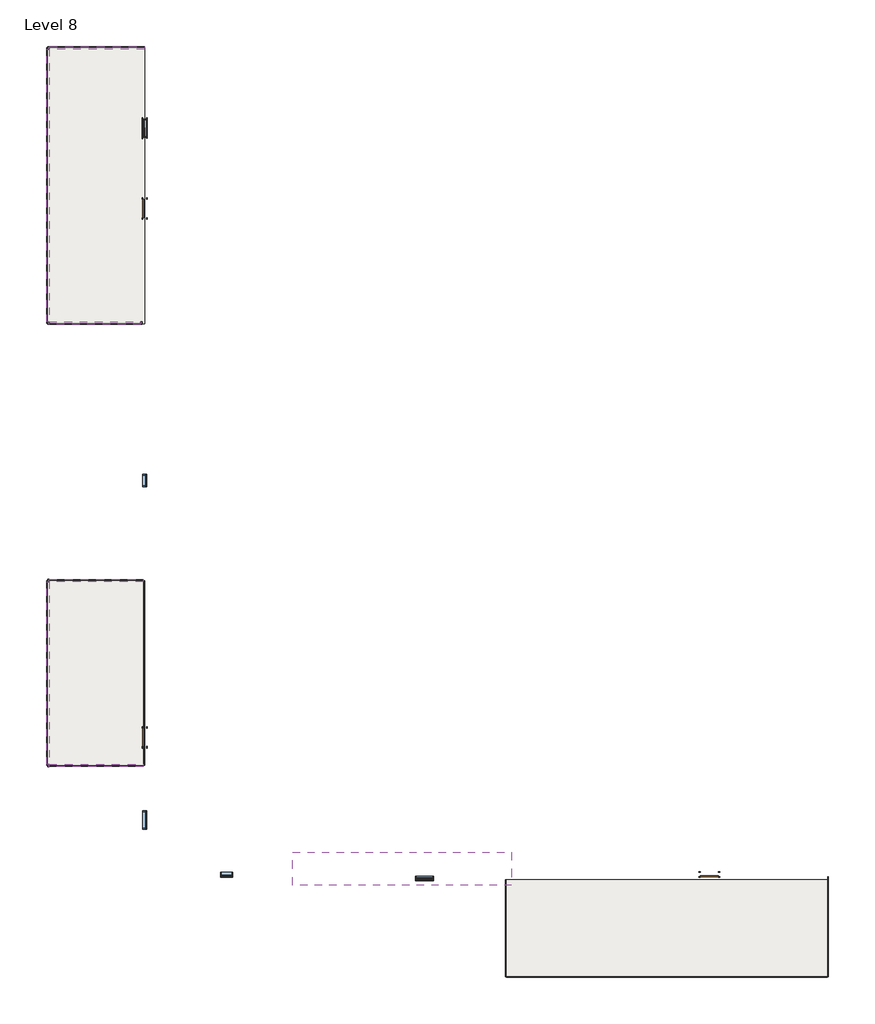
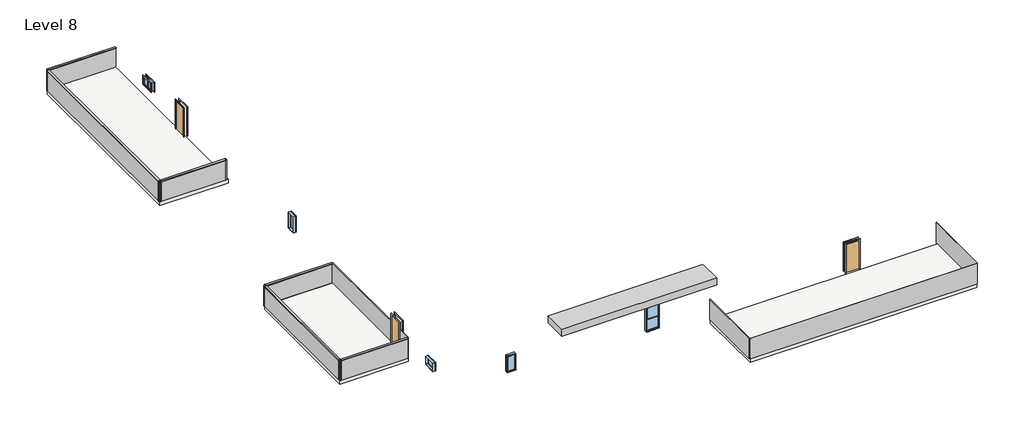
# One storey: 15 members, 10 plates, 5 windows, 3 doors, 3 slabs, 1 proxy.
"""IFC4 building model written with IfcOpenShell, lengths in millimetres."""

from ifc_helpers import new_model, si_unit, frame, origin, place, context, project, spatial, polyline, outline, extrude, transform, mapped, element, save
from components import generic_models_8_generic_models_8_4897e18a, door_54dd4da4, door_719f80de, member_a0ba9e48, member_4491d118, member_ead6e1d0, member_8787ee90, member_3d8465bd, member_a33656d8, system_panel_glazed_6303489a, system_panel_glazed_19389588, system_panel_glazed_29cdcffd, system_panel_glazed_75d2b8fb, system_panel_glazed_82bc3a22, system_panel_glazed_1060ff55, system_panel_glazed_fce9463a, system_panel_glazed_86bade12, system_panel_glazed_21f26c1a, window_f274a882, window_80bd9af0, window_57c3ee1c, window_78885257, window_a4355bb3

model = new_model("IFC4")

# Units and contexts
model_context = context("Model", 3, world=origin())
ifc_project = project(units=[si_unit("LENGTHUNIT", "METRE", prefix="MILLI")], contexts=[model_context])

# Site, building, storey
site = spatial("IfcSite", under=ifc_project)
building = spatial("IfcBuilding", under=site)
storey = spatial("IfcBuildingStorey", under=building, Name="Level 8", Elevation=13106.4)

# Proxy
placement = place(None, origin())
generic_models_8_generic_models_8_shape = generic_models_8_generic_models_8_4897e18a(model_context)
element("IfcBuildingElementProxy", 1, Name="Generic Models 8 : Generic Models 8", ObjectType="Generic Models 8 : Generic Models 8", at=placement, inside=storey, context=model_context, shape_type="MappedRepresentation", body=[
    mapped(generic_models_8_generic_models_8_shape, transform((0.0, 0.0, 0.0), x_axis=(1.0, 0.0, 0.0), y_axis=(0.0, 1.0, 0.0), z_axis=(0.0, 0.0, 1.0))),
])

# Doors
door_shape = door_54dd4da4(model_context)
element("IfcDoor", 2, ObjectType="Single-Flush : 36\" x 84\"", at=placement, inside=storey, context=model_context, shape_type="MappedRepresentation", body=[
    mapped(door_shape, transform((-15175.038074, 12733.0014639, 13106.4), x_axis=(0.0, 1.0, 0.0), y_axis=(-1.0, 0.0, 0.0), z_axis=(0.0, 0.0, 1.0))),
])
element("IfcDoor", 3, ObjectType="Single-Flush : 36\" x 84\"", at=placement, inside=storey, context=model_context, shape_type="MappedRepresentation", body=[
    mapped(door_shape, transform((-15175.038074, -13852.5915889, 13106.4), x_axis=(0.0, 1.0, 0.0), y_axis=(-1.0, 0.0, 0.0), z_axis=(0.0, 0.0, 1.0))),
])
door_2_shape = door_719f80de(model_context)
element("IfcDoor", 4, ObjectType="Single-Flush : 36\" x 84\"", at=placement, inside=storey, context=model_context, shape_type="MappedRepresentation", body=[
    mapped(door_2_shape, transform((13222.161926, -20744.1985361, 13106.4), x_axis=(1.0, 0.0, 0.0), y_axis=(0.0, 1.0, 0.0), z_axis=(0.0, 0.0, 1.0))),
])

# Members
member_shape = member_a0ba9e48(model_context)
element("IfcMember", 5, ObjectType="Rectangular Mullion : 2.5\" x 5\" rectangular", at=placement, inside=storey, context=model_context, shape_type="MappedRepresentation", body=[
    mapped(member_shape, transform((-15175.038074, 20810.2014639, 14630.4), x_axis=(0.0, 0.0, 1.0), y_axis=(0.0, -1.0, 0.0), z_axis=(1.0, 0.0, 0.0))),
])
member_2_shape = member_4491d118(model_context)
element("IfcMember", 6, ObjectType="Rectangular Mullion : 2.5\" x 5\" rectangular", at=placement, inside=storey, context=model_context, shape_type="MappedRepresentation", body=[
    mapped(member_2_shape, transform((-20051.838074, 20810.2014639, 13106.4), x_axis=(0.0, 1.0, 0.0), y_axis=(1.0, 0.0, 0.0), z_axis=(0.0, 0.0, -1.0))),
])
element("IfcMember", 7, ObjectType="Rectangular Mullion : 2.5\" x 5\" rectangular", at=placement, inside=storey, context=model_context, shape_type="MappedRepresentation", body=[
    mapped(member_2_shape, transform((-20051.838074, 6967.2014639, 13106.4), x_axis=(-1.0, 0.0, 0.0), y_axis=(0.0, 1.0, 0.0), z_axis=(0.0, 0.0, -1.0))),
])
element("IfcMember", 8, ObjectType="Rectangular Mullion : 2.5\" x 5\" rectangular", at=placement, inside=storey, context=model_context, shape_type="MappedRepresentation", body=[
    mapped(member_2_shape, transform((-20051.838074, -15263.2213044, 13106.4), x_axis=(-1.0, 0.0, 0.0), y_axis=(0.0, 1.0, 0.0), z_axis=(0.0, 0.0, -1.0))),
])
element("IfcMember", 9, ObjectType="Rectangular Mullion : 2.5\" x 5\" rectangular", at=placement, inside=storey, context=model_context, shape_type="MappedRepresentation", body=[
    mapped(member_2_shape, transform((-20051.838074, -5966.8213044, 13106.4), x_axis=(0.0, 1.0, 0.0), y_axis=(1.0, 0.0, 0.0), z_axis=(0.0, 0.0, -1.0))),
])
element("IfcMember", 10, ObjectType="Rectangular Mullion : 2.5\" x 5\" rectangular", at=placement, inside=storey, context=model_context, shape_type="MappedRepresentation", body=[
    mapped(member_2_shape, transform((-20051.838074, 20810.2014639, 14630.4), x_axis=(-1.0, 0.0, 0.0), y_axis=(0.0, -1.0, 0.0), z_axis=(0.0, 0.0, 1.0))),
])
element("IfcMember", 11, ObjectType="Rectangular Mullion : 2.5\" x 5\" rectangular", at=placement, inside=storey, context=model_context, shape_type="MappedRepresentation", body=[
    mapped(member_2_shape, transform((-20051.838074, 6967.2014639, 14630.4), x_axis=(0.0, -1.0, 0.0), y_axis=(1.0, 0.0, 0.0), z_axis=(0.0, 0.0, 1.0))),
])
element("IfcMember", 12, ObjectType="Rectangular Mullion : 2.5\" x 5\" rectangular", at=placement, inside=storey, context=model_context, shape_type="MappedRepresentation", body=[
    mapped(member_2_shape, transform((-20051.838074, -15263.2213044, 14630.4), x_axis=(0.0, -1.0, 0.0), y_axis=(1.0, 0.0, 0.0), z_axis=(0.0, 0.0, 1.0))),
])
element("IfcMember", 13, ObjectType="Rectangular Mullion : 2.5\" x 5\" rectangular", at=placement, inside=storey, context=model_context, shape_type="MappedRepresentation", body=[
    mapped(member_2_shape, transform((-15308.388074, 6967.2014639, 14630.4), x_axis=(1.0, 0.0, 0.0), y_axis=(0.0, 1.0, 0.0), z_axis=(0.0, 0.0, 1.0))),
])
element("IfcMember", 14, ObjectType="Rectangular Mullion : 2.5\" x 5\" rectangular", at=placement, inside=storey, context=model_context, shape_type="MappedRepresentation", body=[
    mapped(member_2_shape, transform((-20051.838074, -5966.8213044, 14630.4), x_axis=(-1.0, 0.0, 0.0), y_axis=(0.0, -1.0, 0.0), z_axis=(0.0, 0.0, 1.0))),
])
member_3_shape = member_ead6e1d0(model_context)
element("IfcMember", 15, ObjectType="Rectangular Mullion : 2.5\" x 5\" rectangular", at=placement, inside=storey, context=model_context, shape_type="MappedRepresentation", body=[
    mapped(member_3_shape, transform((-20051.838074, 20746.7014639, 14630.4), x_axis=(0.0, 0.0, 1.0), y_axis=(1.0, 0.0, 0.0), z_axis=(0.0, 1.0, 0.0))),
])
member_4_shape = member_8787ee90(model_context)
element("IfcMember", 16, ObjectType="Rectangular Mullion : 2.5\" x 5\" rectangular", at=placement, inside=storey, context=model_context, shape_type="MappedRepresentation", body=[
    mapped(member_4_shape, transform((-20051.838074, -6030.3213044, 14630.4), x_axis=(0.0, 0.0, 1.0), y_axis=(1.0, 0.0, 0.0), z_axis=(0.0, 1.0, 0.0))),
])
member_5_shape = member_3d8465bd(model_context)
element("IfcMember", 17, ObjectType="Rectangular Mullion : 2.5\" x 5\" rectangular", at=placement, inside=storey, context=model_context, shape_type="MappedRepresentation", body=[
    mapped(member_5_shape, transform((-19988.338074, -15263.2213044, 14630.4), x_axis=(0.0, 0.0, 1.0), y_axis=(0.0, 1.0, 0.0), z_axis=(-1.0, 0.0, 0.0))),
])
member_6_shape = member_a33656d8(model_context)
element("IfcMember", 18, ObjectType="Rectangular Mullion : 2.5\" x 5\" rectangular", at=placement, inside=storey, context=model_context, shape_type="MappedRepresentation", body=[
    mapped(member_6_shape, transform((-19988.338074, 6967.2014639, 14630.4), x_axis=(0.0, 0.0, 1.0), y_axis=(0.0, 1.0, 0.0), z_axis=(-1.0, 0.0, 0.0))),
])
element("IfcMember", 19, ObjectType="Rectangular Mullion : 2.5\" x 5\" rectangular", at=placement, inside=storey, context=model_context, shape_type="MappedRepresentation", body=[
    mapped(member_5_shape, transform((-15245.2693425, -5966.8213044, 14630.4), x_axis=(0.0, 0.0, 1.0), y_axis=(0.0, -1.0, 0.0), z_axis=(1.0, 0.0, 0.0))),
])

# Plates
system_panel_glazed_shape = system_panel_glazed_6303489a(model_context)
element("IfcPlate", 20, ObjectType="System Panel : Glazed", at=placement, inside=storey, context=model_context, shape_type="MappedRepresentation", body=[
    mapped(system_panel_glazed_shape, transform((3011.361926, -23436.5985361, 13106.4), x_axis=(0.0, 1.0, 0.0), y_axis=(-1.0, 0.0, 0.0), z_axis=(0.0, 0.0, 1.0))),
])
system_panel_glazed_2_shape = system_panel_glazed_19389588(model_context)
element("IfcPlate", 21, ObjectType="System Panel : Glazed", at=placement, inside=storey, context=model_context, shape_type="MappedRepresentation", body=[
    mapped(system_panel_glazed_2_shape, transform((11085.386926, -25874.9985361, 13106.4), x_axis=(-1.0, 0.0, 0.0), y_axis=(0.0, -1.0, 0.0), z_axis=(0.0, 0.0, 1.0))),
])
system_panel_glazed_3_shape = system_panel_glazed_29cdcffd(model_context)
element("IfcPlate", 22, ObjectType="System Panel : Glazed", at=placement, inside=storey, context=model_context, shape_type="MappedRepresentation", body=[
    mapped(system_panel_glazed_3_shape, transform((19159.411926, -23360.3985361, 13106.4), x_axis=(0.0, -1.0, 0.0), y_axis=(1.0, 0.0, 0.0), z_axis=(0.0, 0.0, 1.0))),
])
system_panel_glazed_4_shape = system_panel_glazed_75d2b8fb(model_context)
element("IfcPlate", 23, ObjectType="System Panel : Glazed", at=placement, inside=storey, context=model_context, shape_type="MappedRepresentation", body=[
    mapped(system_panel_glazed_4_shape, transform((-15245.2693425, -10615.0213044, 13106.4), x_axis=(0.0, -1.0, 0.0), y_axis=(1.0, 0.0, 0.0), z_axis=(0.0, 0.0, 1.0))),
])
system_panel_glazed_5_shape = system_panel_glazed_82bc3a22(model_context)
element("IfcPlate", 24, ObjectType="System Panel : Glazed", at=placement, inside=storey, context=model_context, shape_type="MappedRepresentation", body=[
    mapped(system_panel_glazed_5_shape, transform((-17581.688074, 20810.2014639, 13106.4), x_axis=(1.0, 0.0, 0.0), y_axis=(0.0, 1.0, 0.0), z_axis=(0.0, 0.0, 1.0))),
])
system_panel_glazed_6_shape = system_panel_glazed_1060ff55(model_context)
element("IfcPlate", 25, ObjectType="System Panel : Glazed", at=placement, inside=storey, context=model_context, shape_type="MappedRepresentation", body=[
    mapped(system_panel_glazed_6_shape, transform((-20051.838074, 13888.7014639, 13106.4), x_axis=(0.0, 1.0, 0.0), y_axis=(-1.0, 0.0, 0.0), z_axis=(0.0, 0.0, 1.0))),
])
system_panel_glazed_7_shape = system_panel_glazed_fce9463a(model_context)
element("IfcPlate", 26, ObjectType="System Panel : Glazed", at=placement, inside=storey, context=model_context, shape_type="MappedRepresentation", body=[
    mapped(system_panel_glazed_7_shape, transform((-20051.838074, -10615.0213044, 13106.4), x_axis=(0.0, 1.0, 0.0), y_axis=(-1.0, 0.0, 0.0), z_axis=(0.0, 0.0, 1.0))),
])
system_panel_glazed_8_shape = system_panel_glazed_86bade12(model_context)
element("IfcPlate", 27, ObjectType="System Panel : Glazed", at=placement, inside=storey, context=model_context, shape_type="MappedRepresentation", body=[
    mapped(system_panel_glazed_8_shape, transform((-17616.8037082, -5966.8213044, 13106.4), x_axis=(1.0, 0.0, 0.0), y_axis=(0.0, 1.0, 0.0), z_axis=(0.0, 0.0, 1.0))),
])
element("IfcPlate", 28, ObjectType="System Panel : Glazed", at=placement, inside=storey, context=model_context, shape_type="MappedRepresentation", body=[
    mapped(system_panel_glazed_8_shape, transform((-17616.8037082, -15263.2213044, 13106.4), x_axis=(-1.0, 0.0, 0.0), y_axis=(0.0, -1.0, 0.0), z_axis=(0.0, 0.0, 1.0))),
])
system_panel_glazed_9_shape = system_panel_glazed_21f26c1a(model_context)
element("IfcPlate", 29, ObjectType="System Panel : Glazed", at=placement, inside=storey, context=model_context, shape_type="MappedRepresentation", body=[
    mapped(system_panel_glazed_9_shape, transform((-17680.113074, 6967.2014639, 13106.4), x_axis=(-1.0, 0.0, 0.0), y_axis=(0.0, -1.0, 0.0), z_axis=(0.0, 0.0, 1.0))),
])

# Slabs
element("IfcSlab", 30, ObjectType="Generic - 12\"", at=placement, inside=storey, context=model_context, shape_type="SweptSolid", body=[
    extrude(outline(polyline([(3011.361926, -20998.1985361), (19165.761926, -20998.1985361), (19165.761926, -25874.9985361), (3011.361926, -25874.9985361), (3011.361926, -20998.1985361)])), frame((0.0, 0.0, 12801.6), z_axis=(0.0, 0.0, 1.0), x_axis=(1.0, 0.0, 0.0)), (0.0, 0.0, 1.0), 304.8),
])
element("IfcSlab", 31, ObjectType="Generic - 12\"", at=placement, inside=storey, context=model_context, shape_type="SweptSolid", body=[
    extrude(outline(polyline([(-20051.838074, -15263.2213044), (-20051.838074, -5966.8213044), (-15175.038074, -5966.8213044), (-15175.038074, -15263.2213044), (-20051.838074, -15263.2213044)])), frame((0.0, 0.0, 12801.6), z_axis=(0.0, 0.0, 1.0), x_axis=(1.0, 0.0, 0.0)), (0.0, 0.0, 1.0), 304.8),
])
element("IfcSlab", 32, ObjectType="Generic - 12\"", at=placement, inside=storey, context=model_context, shape_type="SweptSolid", body=[
    extrude(outline(polyline([(-20051.838074, 20810.2014639), (-15175.038074, 20810.2014639), (-15175.038074, 6941.8014639), (-20051.838074, 6941.8014639), (-20051.838074, 20810.2014639)])), frame((0.0, 0.0, 12801.6), z_axis=(0.0, 0.0, 1.0), x_axis=(1.0, 0.0, 0.0)), (0.0, 0.0, 1.0), 304.8),
])

# Windows
window_shape = window_f274a882(model_context)
element("IfcWindow", 33, ObjectType="Double Hung : 36\" x 72\"", at=placement, inside=storey, context=model_context, shape_type="MappedRepresentation", body=[
    mapped(window_shape, transform((-1103.438074, -20921.9985361, 13443.4516227), x_axis=(-1.0, 0.0, 0.0), y_axis=(0.0, -1.0, 0.0), z_axis=(0.0, 0.0, 1.0))),
])
window_2_shape = window_80bd9af0(model_context)
element("IfcWindow", 34, ObjectType="Fixed : 24\" x 48\"", at=placement, inside=storey, context=model_context, shape_type="MappedRepresentation", body=[
    mapped(window_2_shape, transform((-15175.038074, -975.7213044, 13106.4), x_axis=(0.0, -1.0, 0.0), y_axis=(1.0, 0.0, 0.0), z_axis=(0.0, 0.0, 1.0))),
])
window_3_shape = window_57c3ee1c(model_context)
element("IfcWindow", 35, ObjectType="Fixed : 36\" x 24\"", at=placement, inside=storey, context=model_context, shape_type="MappedRepresentation", body=[
    mapped(window_3_shape, transform((-15175.038074, -18041.8099202, 13106.4), x_axis=(0.0, -1.0, 0.0), y_axis=(1.0, 0.0, 0.0), z_axis=(0.0, 0.0, 1.0))),
])
window_4_shape = window_78885257(model_context)
element("IfcWindow", 36, ObjectType="Instance - Fixed : 24\" x 48\"", at=placement, inside=storey, context=model_context, shape_type="MappedRepresentation", body=[
    mapped(window_4_shape, transform((-11098.338074, -20744.1985361, 13106.4), x_axis=(-1.0, 0.0, 0.0), y_axis=(0.0, -1.0, 0.0), z_axis=(0.0, 0.0, 1.0))),
])
window_5_shape = window_a4355bb3(model_context)
element("IfcWindow", 37, ObjectType="Slider with Trim : 36\" x 24\"", at=placement, inside=storey, context=model_context, shape_type="MappedRepresentation", body=[
    mapped(window_5_shape, transform((-15175.038074, 16771.6014639, 13106.4), x_axis=(0.0, 1.0, 0.0), y_axis=(-1.0, 0.0, 0.0), z_axis=(0.0, 0.0, 1.0))),
])

save(model, "model.ifc")

# Revit data of these elements
# Type "Single-Flush : 36\" x 84\""
#   Type Mark = "1"
#   Construction Type Id = "MDOOR"
#   Assembly Code = "C1020"
#   Analytic Construction = "Metal"
#   Thickness = 0' - 2"
#   Heat Transfer Coefficient (U) = 0.651978 BTU/(h·ft²·°F)
#   Height = 7' - 0"
#   Trim Projection Ext = 0' - 1"
#   Trim Projection Int = 0' - 1"
#   Trim Width = 0' - 3"
#   Width = 3' - 0"
#   Define Thermal Properties by = 1
#   Door Material = Door - Panel
#   Frame Material = Door - Frame
#   Visual Light Transmittance = 0
#   Solar Heat Gain Coefficient = 0
#   Function = (empty or 0)
#   Wall Closure = (empty or 0)
# Type "Rectangular Mullion : 2.5\" x 5\" rectangular"
#   built-in parameter 1007304 = 0.416667 (stored number, unit not read)
#   built-in parameter 1007301 = 0.104167 (stored number, unit not read)
#   built-in parameter 1007300 = 0.104167 (stored number, unit not read)
# Type "System Panel : Glazed"
#   Construction Type Id = "GSP4R"
#   Analytic Construction = "1/8 in Pilkington single glazing"
#   Visual Light Transmittance = 0.9
#   Solar Heat Gain Coefficient = 0.86
#   Heat Transfer Coefficient (U) = 1.18115 BTU/(h·ft²·°F)
# Type "Generic - 12\""
#   Assembly Code = "B1010"
#   Function = 0
#   Layers, outside or top first: 1' - 0" no material (function 1)
# Type "Double Hung : 36\" x 72\""
#   Type Mark = "18"
#   Construction Type Id = "GSP4R"
#   Assembly Code = "B2020100"
#   Analytic Construction = "1/8 in Pilkington single glazing"
#   Visual Light Transmittance = 0.9
#   Solar Heat Gain Coefficient = 0.78
#   Heat Transfer Coefficient (U) = 0.6496 BTU/(h·ft²·°F)
#   Height = 6' - 0"
#   Default Sill Height = 1' - 0"
#   Width = 3' - 0"
#   Window Inset = 0' - 0 3/4"
#   Define Thermal Properties by = 1
#   Glass Pane Material = Glass
#   Sash Material = Sash
#   Description = (empty or 0)
#   Wall Closure = (empty or 0)
# Type "Fixed : 24\" x 48\""
#   Type Mark = "2"
#   Construction Type Id = "GSP4R"
#   Assembly Code = "B2020100"
#   Analytic Construction = "1/8 in Pilkington single glazing"
#   Visual Light Transmittance = 0.9
#   Solar Heat Gain Coefficient = 0.78
#   Heat Transfer Coefficient (U) = 0.6496 BTU/(h·ft²·°F)
#   Height = 4' - 0"
#   Default Sill Height = 3' - 0"
#   Width = 2' - 0"
#   Window Inset = 0' - 0 3/4"
#   Define Thermal Properties by = 1
#   Glass Pane Material = Glass
#   Sash Material = Sash
#   Wall Closure = (empty or 0)
# Type "Fixed : 36\" x 24\""
#   Type Mark = "8"
#   Construction Type Id = "GSP4R"
#   Assembly Code = "B2020100"
#   Analytic Construction = "1/8 in Pilkington single glazing"
#   Visual Light Transmittance = 0.9
#   Solar Heat Gain Coefficient = 0.78
#   Heat Transfer Coefficient (U) = 0.6496 BTU/(h·ft²·°F)
#   Height = 2' - 0"
#   Default Sill Height = 3' - 0"
#   Width = 3' - 0"
#   Window Inset = 0' - 0 3/4"
#   Define Thermal Properties by = 1
#   Glass Pane Material = Glass
#   Sash Material = Sash
#   Wall Closure = (empty or 0)
# Type "Instance - Fixed : 24\" x 48\""
#   Type Mark = "19"
#   Construction Type Id = "GSP4R"
#   Assembly Code = "B2020100"
#   Analytic Construction = "1/8 in Pilkington single glazing"
#   Visual Light Transmittance = 0.9
#   Thermal Resistance (R) = 0.8466 (h·ft²·°F)/BTU
#   Solar Heat Gain Coefficient = 0.86
#   Heat Transfer Coefficient (U) = 1.1812 BTU/(h·ft²·°F)
#   Height [instance default] = 4' - 0"
#   Default Sill Height = 3' - 0"
#   Width [instance default] = 2' - 0"
#   Window Inset = 0' - 0 3/4"
#   Define Thermal Properties by = 1
#   Glass Pane Material = Glass
#   Sash Material = Sash
#   Wall Closure = (empty or 0)
# Type "Slider with Trim : 36\" x 24\""
#   Type Mark = "23"
#   Construction Type Id = "GSP4R"
#   Assembly Code = "B2020100"
#   Analytic Construction = "1/8 in Pilkington single glazing"
#   Visual Light Transmittance = 0.9
#   Solar Heat Gain Coefficient = 0.78
#   Heat Transfer Coefficient (U) = 0.6496 BTU/(h·ft²·°F)
#   Height = 2' - 0"
#   Default Sill Height = 3' - 0"
#   Trim Projection - Ext. = 0' - 0 3/4"
#   Trim Projection - Int. = 0' - 0 3/4"
#   Trim Width - Exterior = 0' - 3 1/2"
#   Trim Width - Interior = 0' - 3 1/2"
#   Width = 3' - 0"
#   Window Inset = 0' - 0 3/4"
#   Define Thermal Properties by = 1
#   Glass Pane Material = Glass
#   Sash Material = Sash
#   Trim Exterior Material = Trim
#   Trim Interior Material = Trim
#   Wall Closure = (empty or 0)
# Element 1 (IfcBuildingElementProxy, "Generic Models 8 : Generic Models 8")
#   Phase Created = New Construction
# Elements 2, 3, 4 (IfcDoor, "Single-Flush : 36\" x 84\"")
#   Phase Created = New Construction
#   Materials on its faces: "Door - Frame", "Door - Panel"
# Elements 5, 6, 7, 8, 9, 10, 11, 12, 13, 14, 15, 16, 17, 18, 19 (IfcMember, "Rectangular Mullion : 2.5\" x 5\" rectangular")
#   Phase Created = New Construction
#   Materials on its faces: "Aluminum"
# Elements 20, 21, 22, 23, 24, 25, 26, 27, 28, 29 (IfcPlate, "System Panel : Glazed")
#   Phase Created = New Construction
#   Materials on its faces: "Glass"
# Elements 30, 31, 32 (IfcSlab, "Generic - 12\"")
#   built-in parameter 1001955 = 3.14159 (stored number, unit not read)
#   Height Offset From Level = 0' - 0"
#   Phase Created = New Construction
#   Materials on its faces: "Default Floor"
# Element 33 (IfcWindow, "Double Hung : 36\" x 72\"")
#   Mark = "8"
#   Phase Created = New Construction
#   Materials on its faces: "Sash", "Glass"
# Element 34 (IfcWindow, "Fixed : 24\" x 48\"")
#   Mark = "52"
#   Phase Created = New Construction
#   Materials on its faces: "Sash", "Glass"
# Element 35 (IfcWindow, "Fixed : 36\" x 24\"")
#   Mark = "74"
#   Phase Created = New Construction
#   Materials on its faces: "Sash", "Glass"
# Element 36 (IfcWindow, "Instance - Fixed : 24\" x 48\"")
#   Mark = "19"
#   Width = 2' - 0"
#   Height = 4' - 0"
#   Phase Created = New Construction
#   Materials on its faces: "Sash", "Glass"
# Element 37 (IfcWindow, "Slider with Trim : 36\" x 24\"")
#   Mark = "63"
#   Phase Created = New Construction
#   Materials on its faces: "Sash", "Trim", "Glass"
# Materials
#   "Door - Panel": class "Wood", colour RGB 210 159 95, transparency 0
#   "Door - Frame": colour RGB 118 70 51, transparency 0
#   "Glass": class "Glass", colour RGB 0 128 192, transparency 0.75, Description = "Soda Lime Glass", Cost = 0
#   "Sash": class "Wood", colour RGB 224 178 126, transparency 0
#   "Trim": class "Wood", colour RGB 224 178 126, transparency 0
#   "Aluminum": class "Metal", colour RGB 247 247 247, transparency 0, Description = "Aluminum 6061", Cost = 0
#   "Default Floor": colour RGB 128 128 128, transparency 0
